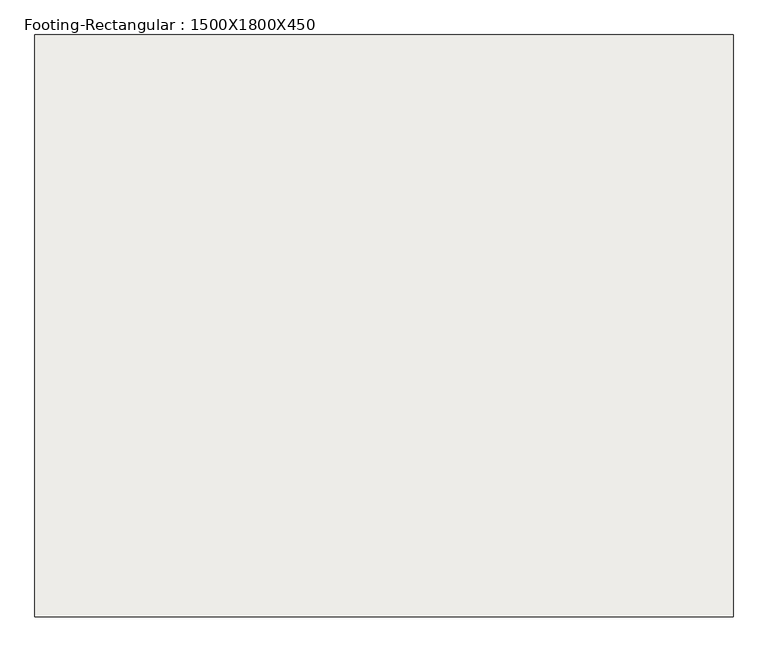
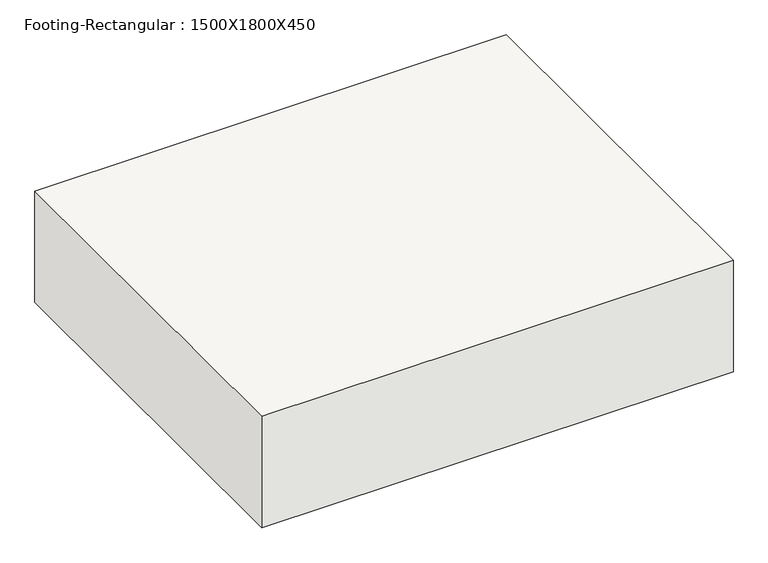
"""IFC4 building model written with IfcOpenShell, lengths in millimetres: slab geometry, Footing-Rectangular : 1500X1800X450."""

from ifc_helpers import new_model, si_unit, frame, origin, place, context, project, spatial, polyline, outline, extrude, source, transform, mapped, element, save


def footing_rectangular_1500x1800x450_b566de6d(model_context):
    return source(origin(), model_context, "Body", "SweptSolid", [
        extrude(outline(polyline([(900.0, 750.0), (900.0, -750.0), (-900.0, -750.0), (-900.0, 750.0), (900.0, 750.0)])), frame((0.0, 0.0, -450.0), z_axis=(0.0, 0.0, 1.0), x_axis=(1.0, 0.0, 0.0)), (0.0, 0.0, 1.0), 450.0),
    ])


if __name__ == "__main__":
    model = new_model("IFC4")
    model_context = context("Model", 3, world=origin())
    ifc_project = project(units=[si_unit("LENGTHUNIT", "METRE", prefix="MILLI")], contexts=[model_context])
    site = spatial("IfcSite", under=ifc_project)
    building = spatial("IfcBuilding", under=site)
    placement = place(None, origin())
    footing_rectangular_1500x1800x450_shape = footing_rectangular_1500x1800x450_b566de6d(model_context)
    element("IfcSlab", 1, ObjectType="Footing-Rectangular : 1500X1800X450", at=placement, inside=building, context=model_context, shape_type="MappedRepresentation", body=[
        mapped(footing_rectangular_1500x1800x450_shape, transform((0.0, 0.0, 0.0), x_axis=(1.0, 0.0, 0.0), y_axis=(0.0, 1.0, 0.0), z_axis=(0.0, 0.0, 1.0))),
    ])
    save(model, "model.ifc")

# Revit data of these elements
# Type "Footing-Rectangular : 1500X1800X450"
#   Width = 5' - 10.86614"
#   Length = 4' - 11.05512"
#   Foundation Thickness = 1' - 5.71654"
#   Structural Material [instance default] = Concrete - Cast-in-Place Concrete
#   Assembly Code = ""
# Element 1 (IfcSlab, "Footing-Rectangular : 1500X1800X450")
#   Materials on its faces: "Concrete - Cast-in-Place Concrete"
# Materials
#   "Concrete - Cast-in-Place Concrete": class "Concrete", colour RGB 192 192 192, transparency 0, Cost = 0
